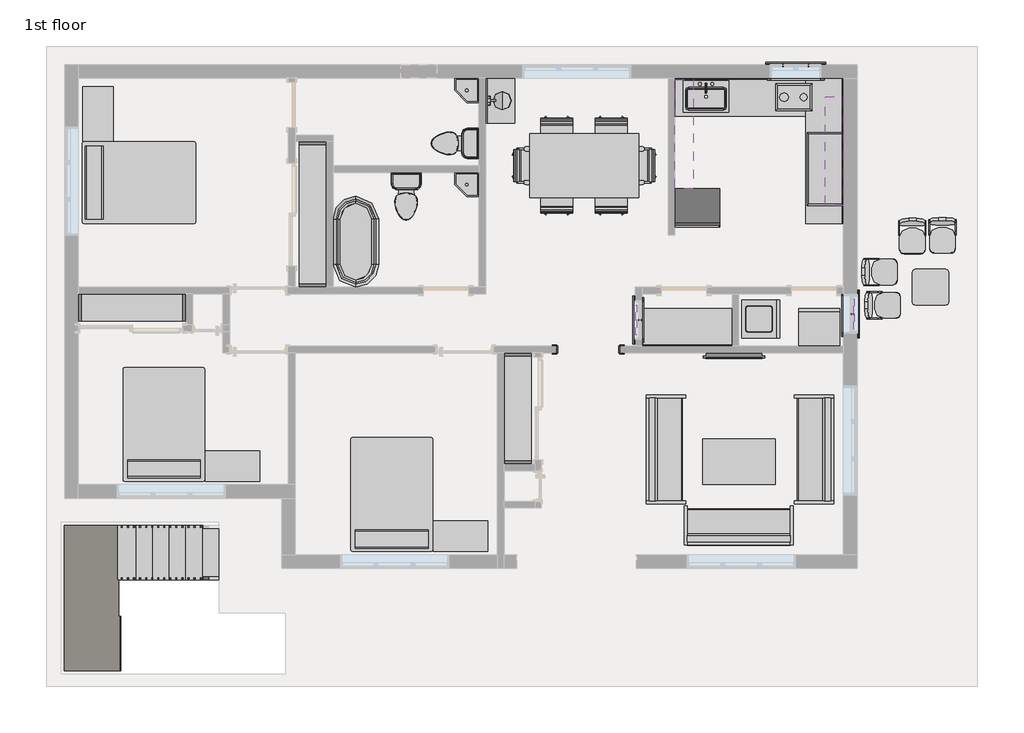
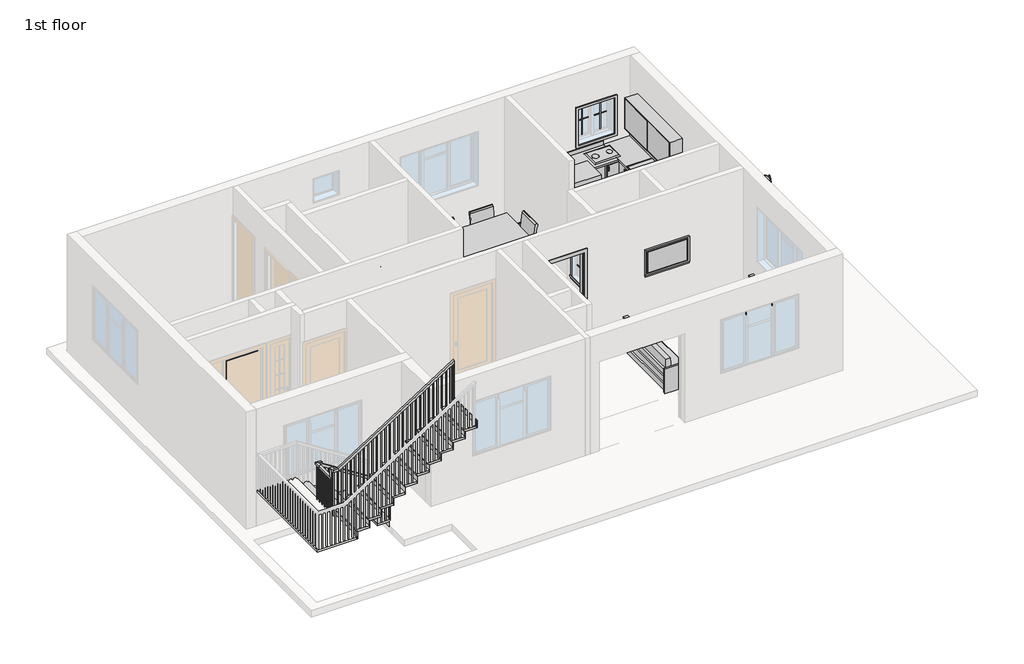
# One storey, part 4 of 4: 34 furniture elements, 17 proxies, 7 flow terminals, 2 stair flights, 1 railing, 1 slab.
"""IFC4 building model written with IfcOpenShell, lengths in millimetres."""

from ifc_helpers import new_model, si_unit, frame, origin, place, context, project, spatial, polyline, outline, extrude, faceted_brep, transform, mapped, element, save
from components import proxy_3c1fa1d0, proxy_97c73763, muntin_pattern_2x2_muntin_pattern_2x2_b3fe6957, muntin_pattern_2x2_muntin_pattern_2x2_3e0ecaf2, muntin_pattern_2x2_muntin_pattern_2x2_c35c595f, muntin_pattern_2x2_muntin_pattern_2x2_183aef24, proxy_bc9927fa, proxy_e6cf46b9, trim_window_exterior_flat_with_sill_41619996, trim_window_exterior_flat_with_sill_e38017c9, trim_window_exterior_flat_with_sill_5e960bf5, trim_window_interior_flat_picture_frame_51c85655, trim_window_interior_flat_picture_frame_d728ed12, trim_window_interior_flat_picture_frame_80babb00, proxy_1934c8a4, flow_terminal_15267b2a, flow_terminal_5b58e753, flow_terminal_4d548711, toilet_domestic_3d_toilet_domestic_3d_ba6479b0, toilet_domestic_3d_toilet_domestic_3d_30431060, flow_terminal_ce36f001, furniture_48488436, furniture_f87f75a4, furniture_97fe820d, furniture_52ef1662, furniture_6b884072, chair_task_chair_task_b7f3823b, chair_task_arms_chair_task_arms_fa5a08ef, furniture_deb1c5d1, furniture_9388d8e7, furniture_74614b7d, furniture_eb3a3c23, furniture_53a00f75, furniture_df918c0e, furniture_57be741f, furniture_57f9710a, furniture_acc2807d, furniture_65ba067b, furniture_5d68651d, furniture_b6aab1a0, furniture_1cc80a06, non_monolithic_landing_2594b9d5, stair_flight_c0af1c60, stair_flight_c577b9fb

model = new_model("IFC4")

# Units and contexts
model_context = context("Model", 3, world=origin())
ifc_project = project(units=[si_unit("LENGTHUNIT", "METRE", prefix="MILLI")], contexts=[model_context])

# Site, building, storey
site = spatial("IfcSite", under=ifc_project)
building = spatial("IfcBuilding", under=site)
storey = spatial("IfcBuildingStorey", under=building, Name="1st floor", Elevation=3810.0)

# Proxies
placement = place(None, origin())
proxy_shape = proxy_3c1fa1d0(model_context)
element("IfcBuildingElementProxy", 1, Name="Cook Top-2 Unit : 12\" x 18\"", ObjectType="Cook Top-2 Unit : 12\" x 18\"", at=placement, inside=storey, context=model_context, shape_type="MappedRepresentation", body=[
    mapped(proxy_shape, transform((3099.7984427, 6060.3661978, 3810.0), x_axis=(0.0, 1.0, 0.0), y_axis=(-1.0, 0.0, 0.0), z_axis=(0.0, 0.0, 1.0))),
])
proxy_2_shape = proxy_97c73763(model_context)
element("IfcBuildingElementProxy", 2, Name="Dryer : 27\" x 25\" x 35\"", ObjectType="Dryer : 27\" x 25\" x 35\"", at=placement, inside=storey, context=model_context, shape_type="MappedRepresentation", body=[
    mapped(proxy_2_shape, transform((3116.0361908, 1961.105194, 3810.0), x_axis=(1.0, 0.0, 0.0), y_axis=(0.0, 1.0, 0.0), z_axis=(0.0, 0.0, 1.0))),
])
muntin_pattern_2x2_muntin_pattern_2x2_shape = muntin_pattern_2x2_muntin_pattern_2x2_b3fe6957(model_context)
element("IfcBuildingElementProxy", 3, Name="Muntin Pattern_2x2 : Muntin Pattern_2x2", ObjectType="Muntin Pattern_2x2 : Muntin Pattern_2x2", at=placement, inside=storey, context=model_context, shape_type="MappedRepresentation", body=[
    mapped(muntin_pattern_2x2_muntin_pattern_2x2_shape, transform((2887.0111471, 6673.1411978, 4972.05), x_axis=(1.0, 0.0, 0.0), y_axis=(0.0, 1.0, 0.0), z_axis=(0.0, 0.0, 1.0))),
])
muntin_pattern_2x2_muntin_pattern_2x2_2_shape = muntin_pattern_2x2_muntin_pattern_2x2_3e0ecaf2(model_context)
element("IfcBuildingElementProxy", 4, Name="Muntin Pattern_2x2 : Muntin Pattern_2x2", ObjectType="Muntin Pattern_2x2 : Muntin Pattern_2x2", at=placement, inside=storey, context=model_context, shape_type="MappedRepresentation", body=[
    mapped(muntin_pattern_2x2_muntin_pattern_2x2_2_shape, transform((3315.6361471, 6673.1411978, 4972.05), x_axis=(-1.0, 0.0, 0.0), y_axis=(0.0, -1.0, 0.0), z_axis=(0.0, 0.0, 1.0))),
])
muntin_pattern_2x2_muntin_pattern_2x2_3_shape = muntin_pattern_2x2_muntin_pattern_2x2_c35c595f(model_context)
element("IfcBuildingElementProxy", 5, Name="Muntin Pattern_2x2 : Muntin Pattern_2x2", ObjectType="Muntin Pattern_2x2 : Muntin Pattern_2x2", at=placement, inside=storey, context=model_context, shape_type="MappedRepresentation", body=[
    mapped(muntin_pattern_2x2_muntin_pattern_2x2_3_shape, transform((4095.0986471, 2498.0161978, 5280.025), x_axis=(0.0, -1.0, 0.0), y_axis=(1.0, 0.0, 0.0), z_axis=(0.0, 0.0, 1.0))),
])
element("IfcBuildingElementProxy", 6, Name="Muntin Pattern_2x2 : Muntin Pattern_2x2", ObjectType="Muntin Pattern_2x2 : Muntin Pattern_2x2", at=placement, inside=storey, context=model_context, shape_type="MappedRepresentation", body=[
    mapped(muntin_pattern_2x2_muntin_pattern_2x2_3_shape, transform((4050.6486471, 2498.0161978, 4800.6), x_axis=(0.0, -1.0, 0.0), y_axis=(1.0, 0.0, 0.0), z_axis=(0.0, 0.0, 1.0))),
])
muntin_pattern_2x2_muntin_pattern_2x2_4_shape = muntin_pattern_2x2_muntin_pattern_2x2_183aef24(model_context)
element("IfcBuildingElementProxy", 7, Name="Muntin Pattern_2x2 : Muntin Pattern_2x2", ObjectType="Muntin Pattern_2x2 : Muntin Pattern_2x2", at=placement, inside=storey, context=model_context, shape_type="MappedRepresentation", body=[
    mapped(muntin_pattern_2x2_muntin_pattern_2x2_4_shape, transform((443.8486471, 2396.4161978, 5280.025), x_axis=(0.0, -1.0, 0.0), y_axis=(1.0, 0.0, 0.0), z_axis=(0.0, 0.0, 1.0))),
])
element("IfcBuildingElementProxy", 8, Name="Muntin Pattern_2x2 : Muntin Pattern_2x2", ObjectType="Muntin Pattern_2x2 : Muntin Pattern_2x2", at=placement, inside=storey, context=model_context, shape_type="MappedRepresentation", body=[
    mapped(muntin_pattern_2x2_muntin_pattern_2x2_4_shape, transform((488.2986471, 2396.4161978, 4800.6), x_axis=(0.0, -1.0, 0.0), y_axis=(1.0, 0.0, 0.0), z_axis=(0.0, 0.0, 1.0))),
])
proxy_3_shape = proxy_bc9927fa(model_context)
element("IfcBuildingElementProxy", 9, Name="Passage Opening-Cased : 36\" x 84\"", ObjectType="Passage Opening-Cased : 36\" x 84\"", at=placement, inside=storey, context=model_context, shape_type="MappedRepresentation", body=[
    mapped(proxy_3_shape, transform((-386.6650096, 1901.1161978, 3810.0), x_axis=(-1.0, 0.0, 0.0), y_axis=(0.0, -1.0, 0.0), z_axis=(0.0, 0.0, 1.0))),
])
proxy_4_shape = proxy_e6cf46b9(model_context)
element("IfcBuildingElementProxy", 10, Name="Refrigerator-Built-in : 30\" x 24\" RH", ObjectType="Refrigerator-Built-in : 30\" x 24\" RH", at=placement, inside=storey, context=model_context, shape_type="MappedRepresentation", body=[
    mapped(proxy_4_shape, transform((1450.3236471, 4309.7422263, 3810.0), x_axis=(1.0, 0.0, 0.0), y_axis=(0.0, 1.0, 0.0), z_axis=(0.0, 0.0, 1.0))),
])
trim_window_exterior_flat_with_sill_shape = trim_window_exterior_flat_with_sill_41619996(model_context)
element("IfcBuildingElementProxy", 11, Name="Trim-Window-Exterior-Flat : with Sill", ObjectType="Trim-Window-Exterior-Flat : with Sill", at=placement, inside=storey, context=model_context, shape_type="MappedRepresentation", body=[
    mapped(trim_window_exterior_flat_with_sill_shape, transform((3101.3236471, 6682.6661978, 5816.6), x_axis=(-1.0, 0.0, 0.0), y_axis=(0.0, 0.0, 1.0), z_axis=(0.0, 1.0, 0.0))),
])
trim_window_exterior_flat_with_sill_2_shape = trim_window_exterior_flat_with_sill_e38017c9(model_context)
element("IfcBuildingElementProxy", 12, Name="Trim-Window-Exterior-Flat : with Sill", ObjectType="Trim-Window-Exterior-Flat : with Sill", at=placement, inside=storey, context=model_context, shape_type="MappedRepresentation", body=[
    mapped(trim_window_exterior_flat_with_sill_2_shape, transform((4130.0236471, 2498.0161978, 5791.2), x_axis=(0.0, 1.0, 0.0), y_axis=(0.0, 0.0, 1.0), z_axis=(1.0, 0.0, 0.0))),
])
trim_window_exterior_flat_with_sill_3_shape = trim_window_exterior_flat_with_sill_5e960bf5(model_context)
element("IfcBuildingElementProxy", 13, Name="Trim-Window-Exterior-Flat : with Sill", ObjectType="Trim-Window-Exterior-Flat : with Sill", at=placement, inside=storey, context=model_context, shape_type="MappedRepresentation", body=[
    mapped(trim_window_exterior_flat_with_sill_3_shape, transform((408.9236471, 2396.4161978, 5791.2), x_axis=(0.0, 1.0, 0.0), y_axis=(0.0, 0.0, -1.0), z_axis=(-1.0, 0.0, 0.0))),
])
trim_window_interior_flat_picture_frame_shape = trim_window_interior_flat_picture_frame_51c85655(model_context)
element("IfcBuildingElementProxy", 14, Name="Trim-Window-Interior-Flat : Picture Frame", ObjectType="Trim-Window-Interior-Flat : Picture Frame", at=placement, inside=storey, context=model_context, shape_type="MappedRepresentation", body=[
    mapped(trim_window_interior_flat_picture_frame_shape, transform((3101.3236471, 6454.0661978, 5816.6), x_axis=(1.0, 0.0, 0.0), y_axis=(0.0, 0.0, 1.0), z_axis=(0.0, -1.0, 0.0))),
])
trim_window_interior_flat_picture_frame_2_shape = trim_window_interior_flat_picture_frame_d728ed12(model_context)
element("IfcBuildingElementProxy", 15, Name="Trim-Window-Interior-Flat : Picture Frame", ObjectType="Trim-Window-Interior-Flat : Picture Frame", at=placement, inside=storey, context=model_context, shape_type="MappedRepresentation", body=[
    mapped(trim_window_interior_flat_picture_frame_2_shape, transform((3901.4236471, 2498.0161978, 5791.2), x_axis=(0.0, -1.0, 0.0), y_axis=(0.0, 0.0, 1.0), z_axis=(-1.0, 0.0, 0.0))),
])
trim_window_interior_flat_picture_frame_3_shape = trim_window_interior_flat_picture_frame_80babb00(model_context)
element("IfcBuildingElementProxy", 16, Name="Trim-Window-Interior-Flat : Picture Frame", ObjectType="Trim-Window-Interior-Flat : Picture Frame", at=placement, inside=storey, context=model_context, shape_type="MappedRepresentation", body=[
    mapped(trim_window_interior_flat_picture_frame_3_shape, transform((523.2236471, 2396.4161978, 5791.2), x_axis=(0.0, -1.0, 0.0), y_axis=(0.0, 0.0, -1.0), z_axis=(1.0, 0.0, 0.0))),
])
proxy_5_shape = proxy_1934c8a4(model_context)
element("IfcBuildingElementProxy", 17, Name="Washer : 25\" x 25\" x 35\"", ObjectType="Washer : 25\" x 25\" x 35\"", at=placement, inside=storey, context=model_context, shape_type="MappedRepresentation", body=[
    mapped(proxy_5_shape, transform((2237.9740823, 2809.1661978, 3810.0), x_axis=(0.0, -1.0, 0.0), y_axis=(1.0, 0.0, 0.0), z_axis=(0.0, 0.0, 1.0))),
])

# Flow terminals
flow_terminal_shape = flow_terminal_15267b2a(model_context)
element("IfcFlowTerminal", 18, ObjectType="Lavatory - Vanity : 30\"x18\" - Private", at=placement, inside=storey, context=model_context, shape_type="MappedRepresentation", body=[
    mapped(flow_terminal_shape, transform((-2099.3263529, 6079.4161978, 3810.0), x_axis=(1.0, 0.0, 0.0), y_axis=(0.0, 1.0, 0.0), z_axis=(0.0, 0.0, 1.0))),
])
flow_terminal_2_shape = flow_terminal_5b58e753(model_context)
element("IfcFlowTerminal", 19, ObjectType="Sink - Mop : 28\"x28\"", at=placement, inside=storey, context=model_context, shape_type="MappedRepresentation", body=[
    mapped(flow_terminal_2_shape, transform((-2213.6263529, 4872.9161978, 3810.0), x_axis=(0.0, -1.0, 0.0), y_axis=(1.0, 0.0, 0.0), z_axis=(0.0, 0.0, 1.0))),
])
element("IfcFlowTerminal", 20, ObjectType="Sink - Mop : 28\"x28\"", at=placement, inside=storey, context=model_context, shape_type="MappedRepresentation", body=[
    mapped(flow_terminal_2_shape, transform((-2213.6263529, 6454.0661978, 3810.0), x_axis=(0.0, -1.0, 0.0), y_axis=(1.0, 0.0, 0.0), z_axis=(0.0, 0.0, 1.0))),
])
flow_terminal_3_shape = flow_terminal_4d548711(model_context)
element("IfcFlowTerminal", 21, ObjectType="Sink Kitchen-Single : 30\" x 21\"", at=placement, inside=storey, context=model_context, shape_type="MappedRepresentation", body=[
    mapped(flow_terminal_3_shape, transform((1580.6844065, 6146.9207967, 3810.0), x_axis=(1.0, 0.0, 0.0), y_axis=(0.0, 1.0, 0.0), z_axis=(0.0, 0.0, 1.0))),
])
toilet_domestic_3d_toilet_domestic_3d_shape = toilet_domestic_3d_toilet_domestic_3d_ba6479b0(model_context)
toilet_domestic_3d_toilet_domestic_3d_2_shape = toilet_domestic_3d_toilet_domestic_3d_30431060(model_context)
element("IfcFlowTerminal", 22, ObjectType="Toilet-Domestic-3D : Toilet-Domestic-3D", at=placement, inside=storey, context=model_context, shape_type="MappedRepresentation", body=[
    mapped(toilet_domestic_3d_toilet_domestic_3d_shape, transform((-3433.7493286, 4378.2201704, 3810.0), x_axis=(1.0, 0.0, 0.0), y_axis=(0.0, 1.0, 0.0), z_axis=(0.0, 0.0, 1.0))),
    mapped(toilet_domestic_3d_toilet_domestic_3d_2_shape, transform((-3433.7493286, 4378.2201704, 3810.0), x_axis=(1.0, 0.0, 0.0), y_axis=(0.0, 1.0, 0.0), z_axis=(0.0, 0.0, 1.0))),
])
element("IfcFlowTerminal", 23, ObjectType="Toilet-Domestic-3D : Toilet-Domestic-3D", at=placement, inside=storey, context=model_context, shape_type="MappedRepresentation", body=[
    mapped(toilet_domestic_3d_toilet_domestic_3d_shape, transform((-2708.3223803, 5361.8661978, 3810.0), x_axis=(0.0, -1.0, 0.0), y_axis=(1.0, 0.0, 0.0), z_axis=(0.0, 0.0, 1.0))),
    mapped(toilet_domestic_3d_toilet_domestic_3d_2_shape, transform((-2708.3223803, 5361.8661978, 3810.0), x_axis=(0.0, -1.0, 0.0), y_axis=(1.0, 0.0, 0.0), z_axis=(0.0, 0.0, 1.0))),
])
flow_terminal_4_shape = flow_terminal_ce36f001(model_context)
element("IfcFlowTerminal", 24, ObjectType="Tub-Free Standing-3D : 30\" x 60\"", at=placement, inside=storey, context=model_context, shape_type="MappedRepresentation", body=[
    mapped(flow_terminal_4_shape, transform((-4277.3763529, 3710.8661978, 3810.0), x_axis=(-1.0, 0.0, 0.0), y_axis=(0.0, -1.0, 0.0), z_axis=(0.0, 0.0, 1.0))),
])

# Furniture
furniture_shape = furniture_48488436(model_context)
element("IfcFurniture", 25, ObjectType="48\"", at=placement, inside=storey, context=model_context, shape_type="MappedRepresentation", body=[
    mapped(furniture_shape, transform((3901.4236471, 5020.9111578, 3810.0), x_axis=(0.0, -1.0, 0.0), y_axis=(1.0, 0.0, 0.0), z_axis=(0.0, 0.0, 1.0))),
])
furniture_2_shape = furniture_f87f75a4(model_context)
element("IfcFurniture", 26, ObjectType="Base Cabinet-Combo01 : 30\"", at=placement, inside=storey, context=model_context, shape_type="MappedRepresentation", body=[
    mapped(furniture_2_shape, transform((2587.2859422, 6454.0661978, 3810.0), x_axis=(1.0, 0.0, 0.0), y_axis=(0.0, 1.0, 0.0), z_axis=(0.0, 0.0, 1.0))),
])
furniture_3_shape = furniture_97fe820d(model_context)
element("IfcFurniture", 27, ObjectType="Base Cabinet-Corner Unit-Square : 36\"", at=placement, inside=storey, context=model_context, shape_type="MappedRepresentation", body=[
    mapped(furniture_3_shape, transform((3374.6859422, 6454.0661978, 3810.0), x_axis=(1.0, 0.0, 0.0), y_axis=(0.0, 1.0, 0.0), z_axis=(0.0, 0.0, 1.0))),
])
furniture_4_shape = furniture_52ef1662(model_context)
element("IfcFurniture", 28, ObjectType="Bed-Standard : Double 54\" x 75\"", at=placement, inside=storey, context=model_context, shape_type="MappedRepresentation", body=[
    mapped(furniture_4_shape, transform((-7961.5214349, 4429.9776732, 3810.0), x_axis=(0.0, 1.0, 0.0), y_axis=(-1.0, 0.0, 0.0), z_axis=(0.0, 0.0, 1.0))),
])
element("IfcFurniture", 29, ObjectType="Bed-Standard : Double 54\" x 75\"", at=placement, inside=storey, context=model_context, shape_type="MappedRepresentation", body=[
    mapped(furniture_4_shape, transform((-7225.3378283, 598.2211158, 3810.0), x_axis=(-1.0, 0.0, 0.0), y_axis=(0.0, -1.0, 0.0), z_axis=(0.0, 0.0, 1.0))),
])
element("IfcFurniture", 30, ObjectType="Bed-Standard : Double 54\" x 75\"", at=placement, inside=storey, context=model_context, shape_type="MappedRepresentation", body=[
    mapped(furniture_4_shape, transform((-3402.6378283, -576.5288842, 3810.0), x_axis=(-1.0, 0.0, 0.0), y_axis=(0.0, -1.0, 0.0), z_axis=(0.0, 0.0, 1.0))),
])
furniture_5_shape = furniture_6b884072(model_context)
element("IfcFurniture", 31, ObjectType="Cabinet File-Lateral 2 Drawer : 36\" x 20\" x 24\"", at=placement, inside=storey, context=model_context, shape_type="MappedRepresentation", body=[
    mapped(furniture_5_shape, transform((-9536.044729, 6037.1887117, 3810.0), x_axis=(0.0, 1.0, 0.0), y_axis=(-1.0, 0.0, 0.0), z_axis=(0.0, 0.0, 1.0))),
])
element("IfcFurniture", 32, ObjectType="Cabinet File-Lateral 2 Drawer : 36\" x 20\" x 24\"", at=placement, inside=storey, context=model_context, shape_type="MappedRepresentation", body=[
    mapped(furniture_5_shape, transform((-6527.4988668, -989.0021783, 3810.0), x_axis=(-1.0, 0.0, 0.0), y_axis=(0.0, -1.0, 0.0), z_axis=(0.0, 0.0, 1.0))),
])
element("IfcFurniture", 33, ObjectType="Cabinet File-Lateral 2 Drawer : 36\" x 20\" x 24\"", at=placement, inside=storey, context=model_context, shape_type="MappedRepresentation", body=[
    mapped(furniture_5_shape, transform((-2698.4488668, -2163.7521783, 3810.0), x_axis=(-1.0, 0.0, 0.0), y_axis=(0.0, -1.0, 0.0), z_axis=(0.0, 0.0, 1.0))),
])
chair_task_chair_task_shape = chair_task_chair_task_b7f3823b(model_context)
element("IfcFurniture", 34, ObjectType="Chair-Task : Chair-Task", at=placement, inside=storey, context=model_context, shape_type="MappedRepresentation", body=[
    mapped(chair_task_chair_task_shape, transform((149.8644668, 5539.5620994, 3810.0), x_axis=(-1.0, 0.0, 0.0), y_axis=(0.0, -1.0, 0.0), z_axis=(0.0, 0.0, 1.0))),
])
element("IfcFurniture", 35, ObjectType="Chair-Task : Chair-Task", at=placement, inside=storey, context=model_context, shape_type="MappedRepresentation", body=[
    mapped(chair_task_chair_task_shape, transform((-132.1171726, 4434.8702962, 3810.0), x_axis=(1.0, 0.0, 0.0), y_axis=(0.0, 1.0, 0.0), z_axis=(0.0, 0.0, 1.0))),
])
element("IfcFurniture", 36, ObjectType="Chair-Task : Chair-Task", at=placement, inside=storey, context=model_context, shape_type="MappedRepresentation", body=[
    mapped(chair_task_chair_task_shape, transform((-764.5355332, 5539.5620994, 3810.0), x_axis=(-1.0, 0.0, 0.0), y_axis=(0.0, -1.0, 0.0), z_axis=(0.0, 0.0, 1.0))),
])
element("IfcFurniture", 37, ObjectType="Chair-Task : Chair-Task", at=placement, inside=storey, context=model_context, shape_type="MappedRepresentation", body=[
    mapped(chair_task_chair_task_shape, transform((-1046.5171726, 4434.8702962, 3810.0), x_axis=(1.0, 0.0, 0.0), y_axis=(0.0, 1.0, 0.0), z_axis=(0.0, 0.0, 1.0))),
])
chair_task_arms_chair_task_arms_shape = chair_task_arms_chair_task_arms_fa5a08ef(model_context)
element("IfcFurniture", 38, ObjectType="Chair-Task Arms : Chair-Task Arms", at=placement, inside=storey, context=model_context, shape_type="MappedRepresentation", body=[
    mapped(chair_task_arms_chair_task_arms_shape, transform((-1381.6722545, 5128.2070175, 3810.0), x_axis=(0.0, -1.0, 0.0), y_axis=(1.0, 0.0, 0.0), z_axis=(0.0, 0.0, 1.0))),
])
element("IfcFurniture", 39, ObjectType="Chair-Task Arms : Chair-Task Arms", at=placement, inside=storey, context=model_context, shape_type="MappedRepresentation", body=[
    mapped(chair_task_arms_chair_task_arms_shape, transform((485.0195487, 4846.2253781, 3810.0), x_axis=(0.0, 1.0, 0.0), y_axis=(-1.0, 0.0, 0.0), z_axis=(0.0, 0.0, 1.0))),
])
furniture_6_shape = furniture_deb1c5d1(model_context)
element("IfcFurniture", 40, ObjectType="Counter Top : 24\" Depth", at=placement, inside=storey, context=model_context, shape_type="MappedRepresentation", body=[
    mapped(furniture_6_shape, transform((3901.4236471, 5253.6039027, 3810.0), x_axis=(0.0, -1.0, 0.0), y_axis=(1.0, 0.0, 0.0), z_axis=(0.0, 0.0, 1.0))),
])
furniture_7_shape = furniture_9388d8e7(model_context)
element("IfcFurniture", 41, ObjectType="Counter Top : 24\" Depth", at=placement, inside=storey, context=model_context, shape_type="MappedRepresentation", body=[
    mapped(furniture_7_shape, transform((834.061352, 1958.2661978, 3810.0), x_axis=(-1.0, 0.0, 0.0), y_axis=(0.0, -1.0, 0.0), z_axis=(0.0, 0.0, 1.0))),
])
furniture_8_shape = furniture_74614b7d(model_context)
element("IfcFurniture", 42, ObjectType="Counter Top w Sink Hole : 24\" Depth", at=placement, inside=storey, context=model_context, shape_type="MappedRepresentation", body=[
    mapped(furniture_8_shape, transform((2276.1359422, 6454.0661978, 3810.0), x_axis=(1.0, 0.0, 0.0), y_axis=(0.0, 1.0, 0.0), z_axis=(0.0, 0.0, 1.0))),
])
furniture_9_shape = furniture_eb3a3c23(model_context)
element("IfcFurniture", 43, ObjectType="Seating-Auditorium : 18\" x 24\" x 30\"", at=placement, inside=storey, context=model_context, shape_type="MappedRepresentation", body=[
    mapped(furniture_9_shape, transform((4308.4482373, 3363.5940666, 3810.0), x_axis=(0.0, -1.0, 0.0), y_axis=(1.0, 0.0, 0.0), z_axis=(0.0, 0.0, 1.0))),
])
element("IfcFurniture", 44, ObjectType="Seating-Auditorium : 18\" x 24\" x 30\"", at=placement, inside=storey, context=model_context, shape_type="MappedRepresentation", body=[
    mapped(furniture_9_shape, transform((4359.2482373, 2804.7940666, 3810.0), x_axis=(0.0, -1.0, 0.0), y_axis=(1.0, 0.0, 0.0), z_axis=(0.0, 0.0, 1.0))),
])
element("IfcFurniture", 45, ObjectType="Seating-Auditorium : 18\" x 24\" x 30\"", at=placement, inside=storey, context=model_context, shape_type="MappedRepresentation", body=[
    mapped(furniture_9_shape, transform((5217.8515159, 4002.3416076, 3810.0), x_axis=(-1.0, 0.0, 0.0), y_axis=(0.0, -1.0, 0.0), z_axis=(0.0, 0.0, 1.0))),
])
element("IfcFurniture", 46, ObjectType="Seating-Auditorium : 18\" x 24\" x 30\"", at=placement, inside=storey, context=model_context, shape_type="MappedRepresentation", body=[
    mapped(furniture_9_shape, transform((5725.8515159, 4015.0416076, 3810.0), x_axis=(-1.0, 0.0, 0.0), y_axis=(0.0, -1.0, 0.0), z_axis=(0.0, 0.0, 1.0))),
])
furniture_10_shape = furniture_53a00f75(model_context)
element("IfcFurniture", 47, ObjectType="Shelving : 96\" x 12\" x 84\"", at=placement, inside=storey, context=model_context, shape_type="MappedRepresentation", body=[
    mapped(furniture_10_shape, transform((-1864.3763529, 910.5161978, 3810.0), x_axis=(0.0, 1.0, 0.0), y_axis=(-1.0, 0.0, 0.0), z_axis=(0.0, 0.0, 1.0))),
])
furniture_11_shape = furniture_df918c0e(model_context)
element("IfcFurniture", 48, ObjectType="Shelving : 96\" x 12\" x 84\" 2", at=placement, inside=storey, context=model_context, shape_type="MappedRepresentation", body=[
    mapped(furniture_11_shape, transform((-8030.2263529, 2910.7661978, 3810.0), x_axis=(1.0, 0.0, 0.0), y_axis=(0.0, 1.0, 0.0), z_axis=(0.0, 0.0, 1.0))),
])
furniture_12_shape = furniture_57be741f(model_context)
element("IfcFurniture", 49, ObjectType="Shelving : 96\" x 12\" x 84\" 3", at=placement, inside=storey, context=model_context, shape_type="MappedRepresentation", body=[
    mapped(furniture_12_shape, transform((-5306.0763529, 4168.0661978, 3810.0), x_axis=(0.0, 1.0, 0.0), y_axis=(-1.0, 0.0, 0.0), z_axis=(0.0, 0.0, 1.0))),
])
furniture_13_shape = furniture_57f9710a(model_context)
element("IfcFurniture", 50, ObjectType="Sofa : 72\"", at=placement, inside=storey, context=model_context, shape_type="MappedRepresentation", body=[
    mapped(furniture_13_shape, transform((2219.1941389, -905.4797038, 3810.0), x_axis=(-1.0, 0.0, 0.0), y_axis=(0.0, -1.0, 0.0), z_axis=(0.0, 0.0, 1.0))),
])
element("IfcFurniture", 51, ObjectType="Sofa : 72\"", at=placement, inside=storey, context=model_context, shape_type="MappedRepresentation", body=[
    mapped(furniture_13_shape, transform((3259.9695487, 295.0866896, 3810.0), x_axis=(0.0, -1.0, 0.0), y_axis=(1.0, 0.0, 0.0), z_axis=(0.0, 0.0, 1.0))),
])
element("IfcFurniture", 52, ObjectType="Sofa : 72\"", at=placement, inside=storey, context=model_context, shape_type="MappedRepresentation", body=[
    mapped(furniture_13_shape, transform((1069.4277455, 154.345706, 3810.0), x_axis=(0.0, 1.0, 0.0), y_axis=(-1.0, 0.0, 0.0), z_axis=(0.0, 0.0, 1.0))),
])
furniture_14_shape = furniture_acc2807d(model_context)
element("IfcFurniture", 53, ObjectType="Table-Coffee Rectangular : 48\" x 30\"", at=placement, inside=storey, context=model_context, shape_type="MappedRepresentation", body=[
    mapped(furniture_14_shape, transform((1535.4900168, -354.444634, 3810.0), x_axis=(1.0, 0.0, 0.0), y_axis=(0.0, 1.0, 0.0), z_axis=(0.0, 0.0, 1.0))),
])
furniture_15_shape = furniture_65ba067b(model_context)
element("IfcFurniture", 54, ObjectType="Table-Conference2 w Chairs : 40\" x 90\"", at=placement, inside=storey, context=model_context, shape_type="MappedRepresentation", body=[
    mapped(furniture_15_shape, transform((-448.3263529, 4987.2161978, 3810.0), x_axis=(1.0, 0.0, 0.0), y_axis=(0.0, 1.0, 0.0), z_axis=(0.0, 0.0, 1.0))),
])
furniture_16_shape = furniture_5d68651d(model_context)
element("IfcFurniture", 55, ObjectType="Table-End : 24\" x 24\"", at=placement, inside=storey, context=model_context, shape_type="MappedRepresentation", body=[
    mapped(furniture_16_shape, transform((5053.3900168, 2796.4661978, 3810.0), x_axis=(1.0, 0.0, 0.0), y_axis=(0.0, 1.0, 0.0), z_axis=(0.0, 0.0, 1.0))),
])
furniture_17_shape = furniture_b6aab1a0(model_context)
element("IfcFurniture", 56, ObjectType="Television-Plasma : 42\"", at=placement, inside=storey, context=model_context, shape_type="MappedRepresentation", body=[
    mapped(furniture_17_shape, transform((2009.1236471, 1843.9661978, 4876.8), x_axis=(1.0, 0.0, 0.0), y_axis=(0.0, 1.0, 0.0), z_axis=(0.0, 0.0, 1.0))),
])
furniture_18_shape = furniture_1cc80a06(model_context)
element("IfcFurniture", 57, ObjectType="Upper Cabinet-Pass-Thru w Glass : 48\" x 30\" x 12\"", at=placement, inside=storey, context=model_context, shape_type="MappedRepresentation", body=[
    mapped(furniture_18_shape, transform((1075.6736471, 5495.5284929, 3810.0), x_axis=(0.0, 1.0, 0.0), y_axis=(-1.0, 0.0, 0.0), z_axis=(0.0, 0.0, 1.0))),
])
element("IfcFurniture", 58, ObjectType="Upper Cabinet-Pass-Thru w Glass : 48\" x 30\" x 12\"", at=placement, inside=storey, context=model_context, shape_type="MappedRepresentation", body=[
    mapped(furniture_18_shape, transform((3596.6236471, 5216.1284929, 3810.0), x_axis=(0.0, 1.0, 0.0), y_axis=(-1.0, 0.0, 0.0), z_axis=(0.0, 0.0, 1.0))),
])

# Railing
element("IfcRailing", 59, ObjectType="Handrail - Rectangular", at=placement, inside=storey, context=model_context, shape_type="SolidModel", body=[
    faceted_brep([(-6576.0763529, -1966.0338022, 4902.2), (-6576.0763529, -1966.0338022, 4841.986276), (-6576.0763529, -1915.2338022, 4841.986276), (-6576.0763529, -1915.2338022, 4902.2), (-8176.2763529, -1966.0338022, 5920.5090909), (-8227.0763529, -1966.0338022, 5892.6226396), (-8227.0763529, -1915.2338022, 5892.6226396), (-8176.2763529, -1915.2338022, 5920.5090909), (-8176.2763529, -1966.0338022, 5969.0), (-8227.0763529, -1966.0338022, 5918.2), (-8227.0763529, -1915.2338022, 5918.2), (-8176.2763529, -1915.2338022, 5969.0), (-8252.4763529, -1966.0338022, 5969.0), (-8252.4763529, -1966.0338022, 5918.2), (-8303.2763529, -1915.2338022, 5918.2), (-8303.2763529, -1915.2338022, 5969.0), (-8252.4763529, -2042.2338022, 5969.0), (-8252.4763529, -2042.2338022, 5918.2), (-8303.2763529, -2042.2338022, 5918.2), (-8303.2763529, -2042.2338022, 5969.0), (-8252.4763529, -2499.4338022, 5969.0), (-8252.4763529, -2550.2338022, 5918.2), (-8303.2763529, -2550.2338022, 5918.2), (-8303.2763529, -2499.4338022, 5969.0), (-8252.4763529, -2499.4338022, 6195.2909091), (-8252.4763529, -2550.2338022, 6144.4909091), (-8303.2763529, -2550.2338022, 6144.4909091), (-8303.2763529, -2499.4338022, 6195.2909091), (-8252.4763529, -2575.6338022, 6195.2909091), (-8252.4763529, -2575.6338022, 6144.4909091), (-8303.2763529, -2626.4338022, 6144.4909091), (-8303.2763529, -2626.4338022, 6195.2909091), (-8176.2763529, -2575.6338022, 6195.2909091), (-8161.483358, -2575.6338022, 6144.4909091), (-8161.483358, -2626.4338022, 6144.4909091), (-8176.2763529, -2626.4338022, 6195.2909091), (-5458.4763529, -2575.6338022, 7924.8), (-5458.4763529, -2626.4338022, 7924.8), (-5458.4763529, -2626.4338022, 7864.586276), (-5458.4763529, -2575.6338022, 7864.586276)], [[[0, 1, 2, 3]], [[1, 0, 4, 5]], [[2, 1, 5, 6]], [[3, 2, 6, 7]], [[0, 3, 7, 4]], [[5, 4, 8, 9]], [[6, 5, 9, 10]], [[7, 6, 10, 11]], [[4, 7, 11, 8]], [[9, 8, 12, 13]], [[10, 9, 13, 14]], [[11, 10, 14, 15]], [[8, 11, 15, 12]], [[13, 12, 16, 17]], [[14, 13, 17, 18]], [[15, 14, 18, 19]], [[12, 15, 19, 16]], [[17, 16, 20, 21]], [[18, 17, 21, 22]], [[19, 18, 22, 23]], [[16, 19, 23, 20]], [[21, 20, 24, 25]], [[22, 21, 25, 26]], [[23, 22, 26, 27]], [[20, 23, 27, 24]], [[25, 24, 28, 29]], [[26, 25, 29, 30]], [[27, 26, 30, 31]], [[24, 27, 31, 28]], [[29, 28, 32, 33]], [[30, 29, 33, 34]], [[31, 30, 34, 35]], [[28, 31, 35, 32]], [[36, 37, 38, 39]], [[33, 32, 36, 39]], [[34, 33, 39, 38]], [[35, 34, 38, 37]], [[32, 35, 37, 36]]]),
    extrude(outline(polyline([(7810.0340032, -5544.2013529), (6832.6, -5544.2013529), (6832.6, -5525.1513529), (7822.1567305, -5525.1513529), (7810.0340032, -5544.2013529)])), frame((0.0, -2610.5588022, 0.0), z_axis=(0.0, 1.0, 0.0), x_axis=(0.0, 0.0, 1.0)), (0.0, 0.0, 1.0), 19.05),
    extrude(outline(polyline([(7745.3794578, -5645.8013529), (6832.6, -5645.8013529), (6832.6, -5626.7513529), (7757.5021851, -5626.7513529), (7745.3794578, -5645.8013529)])), frame((0.0, -2610.5588022, 0.0), z_axis=(0.0, 1.0, 0.0), x_axis=(0.0, 0.0, 1.0)), (0.0, 0.0, 1.0), 19.05),
    extrude(outline(polyline([(7680.7249123, -5747.4013529), (6832.6, -5747.4013529), (6832.6, -5728.3513529), (7692.8476396, -5728.3513529), (7680.7249123, -5747.4013529)])), frame((0.0, -2610.5588022, 0.0), z_axis=(0.0, 1.0, 0.0), x_axis=(0.0, 0.0, 1.0)), (0.0, 0.0, 1.0), 19.05),
    extrude(outline(polyline([(7616.0703669, -5849.0013529), (6654.8, -5849.0013529), (6654.8, -5829.9513529), (7628.1930941, -5829.9513529), (7616.0703669, -5849.0013529)])), frame((0.0, -2610.5588022, 0.0), z_axis=(0.0, 1.0, 0.0), x_axis=(0.0, 0.0, 1.0)), (0.0, 0.0, 1.0), 19.05),
    extrude(outline(polyline([(7551.4158214, -5950.6013529), (6654.8, -5950.6013529), (6654.8, -5931.5513529), (7563.5385487, -5931.5513529), (7551.4158214, -5950.6013529)])), frame((0.0, -2610.5588022, 0.0), z_axis=(0.0, 1.0, 0.0), x_axis=(0.0, 0.0, 1.0)), (0.0, 0.0, 1.0), 19.05),
    extrude(outline(polyline([(7486.761276, -6052.2013529), (6477.0, -6052.2013529), (6477.0, -6033.1513529), (7498.8840032, -6033.1513529), (7486.761276, -6052.2013529)])), frame((0.0, -2610.5588022, 0.0), z_axis=(0.0, 1.0, 0.0), x_axis=(0.0, 0.0, 1.0)), (0.0, 0.0, 1.0), 19.05),
    extrude(outline(polyline([(7422.1067305, -6153.8013529), (6477.0, -6153.8013529), (6477.0, -6134.7513529), (7434.2294578, -6134.7513529), (7422.1067305, -6153.8013529)])), frame((0.0, -2610.5588022, 0.0), z_axis=(0.0, 1.0, 0.0), x_axis=(0.0, 0.0, 1.0)), (0.0, 0.0, 1.0), 19.05),
    extrude(outline(polyline([(7357.4521851, -6255.4013529), (6477.0, -6255.4013529), (6477.0, -6236.3513529), (7369.5749123, -6236.3513529), (7357.4521851, -6255.4013529)])), frame((0.0, -2610.5588022, 0.0), z_axis=(0.0, 1.0, 0.0), x_axis=(0.0, 0.0, 1.0)), (0.0, 0.0, 1.0), 19.05),
    extrude(outline(polyline([(7292.7976396, -6357.0013529), (6299.2, -6357.0013529), (6299.2, -6337.9513529), (7304.9203669, -6337.9513529), (7292.7976396, -6357.0013529)])), frame((0.0, -2610.5588022, 0.0), z_axis=(0.0, 1.0, 0.0), x_axis=(0.0, 0.0, 1.0)), (0.0, 0.0, 1.0), 19.05),
    extrude(outline(polyline([(7228.1430941, -6458.6013529), (6299.2, -6458.6013529), (6299.2, -6439.5513529), (7240.2658214, -6439.5513529), (7228.1430941, -6458.6013529)])), frame((0.0, -2610.5588022, 0.0), z_axis=(0.0, 1.0, 0.0), x_axis=(0.0, 0.0, 1.0)), (0.0, 0.0, 1.0), 19.05),
    extrude(outline(polyline([(7163.4885487, -6560.2013529), (6299.2, -6560.2013529), (6299.2, -6541.1513529), (7175.611276, -6541.1513529), (7163.4885487, -6560.2013529)])), frame((0.0, -2610.5588022, 0.0), z_axis=(0.0, 1.0, 0.0), x_axis=(0.0, 0.0, 1.0)), (0.0, 0.0, 1.0), 19.05),
    extrude(outline(polyline([(7098.8340032, -6661.8013529), (6121.4, -6661.8013529), (6121.4, -6642.7513529), (7110.9567305, -6642.7513529), (7098.8340032, -6661.8013529)])), frame((0.0, -2610.5588022, 0.0), z_axis=(0.0, 1.0, 0.0), x_axis=(0.0, 0.0, 1.0)), (0.0, 0.0, 1.0), 19.05),
    extrude(outline(polyline([(7034.1794578, -6763.4013529), (6121.4, -6763.4013529), (6121.4, -6744.3513529), (7046.3021851, -6744.3513529), (7034.1794578, -6763.4013529)])), frame((0.0, -2610.5588022, 0.0), z_axis=(0.0, 1.0, 0.0), x_axis=(0.0, 0.0, 1.0)), (0.0, 0.0, 1.0), 19.05),
    extrude(outline(polyline([(6969.5249123, -6865.0013529), (6121.4, -6865.0013529), (6121.4, -6845.9513529), (6981.6476396, -6845.9513529), (6969.5249123, -6865.0013529)])), frame((0.0, -2610.5588022, 0.0), z_axis=(0.0, 1.0, 0.0), x_axis=(0.0, 0.0, 1.0)), (0.0, 0.0, 1.0), 19.05),
    extrude(outline(polyline([(6904.8703669, -6966.6013529), (5943.6, -6966.6013529), (5943.6, -6947.5513529), (6916.9930941, -6947.5513529), (6904.8703669, -6966.6013529)])), frame((0.0, -2610.5588022, 0.0), z_axis=(0.0, 1.0, 0.0), x_axis=(0.0, 0.0, 1.0)), (0.0, 0.0, 1.0), 19.05),
    extrude(outline(polyline([(6840.2158214, -7068.2013529), (5943.6, -7068.2013529), (5943.6, -7049.1513529), (6852.3385487, -7049.1513529), (6840.2158214, -7068.2013529)])), frame((0.0, -2610.5588022, 0.0), z_axis=(0.0, 1.0, 0.0), x_axis=(0.0, 0.0, 1.0)), (0.0, 0.0, 1.0), 19.05),
    extrude(outline(polyline([(6775.561276, -7169.8013529), (5765.8, -7169.8013529), (5765.8, -7150.7513529), (6787.6840032, -7150.7513529), (6775.561276, -7169.8013529)])), frame((0.0, -2610.5588022, 0.0), z_axis=(0.0, 1.0, 0.0), x_axis=(0.0, 0.0, 1.0)), (0.0, 0.0, 1.0), 19.05),
    extrude(outline(polyline([(6710.9067305, -7271.4013529), (5765.8, -7271.4013529), (5765.8, -7252.3513529), (6723.0294578, -7252.3513529), (6710.9067305, -7271.4013529)])), frame((0.0, -2610.5588022, 0.0), z_axis=(0.0, 1.0, 0.0), x_axis=(0.0, 0.0, 1.0)), (0.0, 0.0, 1.0), 19.05),
    extrude(outline(polyline([(6646.2521851, -7373.0013529), (5765.8, -7373.0013529), (5765.8, -7353.9513529), (6658.3749123, -7353.9513529), (6646.2521851, -7373.0013529)])), frame((0.0, -2610.5588022, 0.0), z_axis=(0.0, 1.0, 0.0), x_axis=(0.0, 0.0, 1.0)), (0.0, 0.0, 1.0), 19.05),
    extrude(outline(polyline([(6581.5976396, -7474.6013529), (5588.0, -7474.6013529), (5588.0, -7455.5513529), (6593.7203669, -7455.5513529), (6581.5976396, -7474.6013529)])), frame((0.0, -2610.5588022, 0.0), z_axis=(0.0, 1.0, 0.0), x_axis=(0.0, 0.0, 1.0)), (0.0, 0.0, 1.0), 19.05),
    extrude(outline(polyline([(6516.9430941, -7576.2013529), (5588.0, -7576.2013529), (5588.0, -7557.1513529), (6529.0658214, -7557.1513529), (6516.9430941, -7576.2013529)])), frame((0.0, -2610.5588022, 0.0), z_axis=(0.0, 1.0, 0.0), x_axis=(0.0, 0.0, 1.0)), (0.0, 0.0, 1.0), 19.05),
    extrude(outline(polyline([(6452.2885487, -7677.8013529), (5588.0, -7677.8013529), (5588.0, -7658.7513529), (6464.411276, -7658.7513529), (6452.2885487, -7677.8013529)])), frame((0.0, -2610.5588022, 0.0), z_axis=(0.0, 1.0, 0.0), x_axis=(0.0, 0.0, 1.0)), (0.0, 0.0, 1.0), 19.05),
    extrude(outline(polyline([(6387.6340032, -7779.4013529), (5410.2, -7779.4013529), (5410.2, -7760.3513529), (6399.7567305, -7760.3513529), (6387.6340032, -7779.4013529)])), frame((0.0, -2610.5588022, 0.0), z_axis=(0.0, 1.0, 0.0), x_axis=(0.0, 0.0, 1.0)), (0.0, 0.0, 1.0), 19.05),
    extrude(outline(polyline([(6322.9794578, -7881.0013529), (5410.2, -7881.0013529), (5410.2, -7861.9513529), (6335.1021851, -7861.9513529), (6322.9794578, -7881.0013529)])), frame((0.0, -2610.5588022, 0.0), z_axis=(0.0, 1.0, 0.0), x_axis=(0.0, 0.0, 1.0)), (0.0, 0.0, 1.0), 19.05),
    extrude(outline(polyline([(6258.3249123, -7982.6013529), (5410.2, -7982.6013529), (5410.2, -7963.5513529), (6270.4476396, -7963.5513529), (6258.3249123, -7982.6013529)])), frame((0.0, -2610.5588022, 0.0), z_axis=(0.0, 1.0, 0.0), x_axis=(0.0, 0.0, 1.0)), (0.0, 0.0, 1.0), 19.05),
    extrude(outline(polyline([(6193.6703669, -8084.2013529), (5232.4, -8084.2013529), (5232.4, -8065.1513529), (6205.7930941, -8065.1513529), (6193.6703669, -8084.2013529)])), frame((0.0, -2610.5588022, 0.0), z_axis=(0.0, 1.0, 0.0), x_axis=(0.0, 0.0, 1.0)), (0.0, 0.0, 1.0), 19.05),
    extrude(outline(polyline([(6129.0158214, -8185.8013529), (5232.4, -8185.8013529), (5232.4, -8166.7513529), (6141.1385487, -8166.7513529), (6129.0158214, -8185.8013529)])), frame((0.0, -2610.5588022, 0.0), z_axis=(0.0, 1.0, 0.0), x_axis=(0.0, 0.0, 1.0)), (0.0, 0.0, 1.0), 19.05),
    extrude(outline(polyline([(-8268.3513529, -2540.7088022), (-8268.3513529, -2559.7588022), (-8287.4013529, -2559.7588022), (-8287.4013529, -2540.7088022), (-8268.3513529, -2540.7088022)])), frame((0.0, 0.0, 5054.6), z_axis=(0.0, 0.0, 1.0), x_axis=(1.0, 0.0, 0.0)), (0.0, 0.0, 1.0), 1089.8909091),
    extrude(outline(polyline([(-8268.3513529, -2439.1088022), (-8268.3513529, -2458.1588022), (-8287.4013529, -2458.1588022), (-8287.4013529, -2439.1088022), (-8268.3513529, -2439.1088022)])), frame((0.0, 0.0, 5054.6), z_axis=(0.0, 0.0, 1.0), x_axis=(1.0, 0.0, 0.0)), (0.0, 0.0, 1.0), 863.6),
    extrude(outline(polyline([(-8268.3513529, -2337.5088022), (-8268.3513529, -2356.5588022), (-8287.4013529, -2356.5588022), (-8287.4013529, -2337.5088022), (-8268.3513529, -2337.5088022)])), frame((0.0, 0.0, 5054.6), z_axis=(0.0, 0.0, 1.0), x_axis=(1.0, 0.0, 0.0)), (0.0, 0.0, 1.0), 863.6),
    extrude(outline(polyline([(-8268.3513529, -2235.9088022), (-8268.3513529, -2254.9588022), (-8287.4013529, -2254.9588022), (-8287.4013529, -2235.9088022), (-8268.3513529, -2235.9088022)])), frame((0.0, 0.0, 5054.6), z_axis=(0.0, 0.0, 1.0), x_axis=(1.0, 0.0, 0.0)), (0.0, 0.0, 1.0), 863.6),
    extrude(outline(polyline([(-8268.3513529, -2134.3088022), (-8268.3513529, -2153.3588022), (-8287.4013529, -2153.3588022), (-8287.4013529, -2134.3088022), (-8268.3513529, -2134.3088022)])), frame((0.0, 0.0, 5054.6), z_axis=(0.0, 0.0, 1.0), x_axis=(1.0, 0.0, 0.0)), (0.0, 0.0, 1.0), 863.6),
    extrude(outline(polyline([(-8268.3513529, -2032.7088022), (-8268.3513529, -2051.7588022), (-8287.4013529, -2051.7588022), (-8287.4013529, -2032.7088022), (-8268.3513529, -2032.7088022)])), frame((0.0, 0.0, 5054.6), z_axis=(0.0, 0.0, 1.0), x_axis=(1.0, 0.0, 0.0)), (0.0, 0.0, 1.0), 863.6),
    extrude(outline(polyline([(-8192.1513529, -1950.1588022), (-8211.2013529, -1950.1588022), (-8211.2013529, -1931.1088022), (-8192.1513529, -1931.1088022), (-8192.1513529, -1950.1588022)])), frame((0.0, 0.0, 4876.8), z_axis=(0.0, 0.0, 1.0), x_axis=(1.0, 0.0, 0.0)), (0.0, 0.0, 1.0), 1041.4),
    extrude(outline(polyline([(5817.8658214, -8109.6013529), (4876.8, -8109.6013529), (4876.8, -8090.5513529), (5805.7430941, -8090.5513529), (5817.8658214, -8109.6013529)])), frame((0.0, -1950.1588022, 0.0), z_axis=(0.0, 1.0, 0.0), x_axis=(0.0, 0.0, 1.0)), (0.0, 0.0, 1.0), 19.05),
    extrude(outline(polyline([(5753.211276, -8008.0013529), (4876.8, -8008.0013529), (4876.8, -7988.9513529), (5741.0885487, -7988.9513529), (5753.211276, -8008.0013529)])), frame((0.0, -1950.1588022, 0.0), z_axis=(0.0, 1.0, 0.0), x_axis=(0.0, 0.0, 1.0)), (0.0, 0.0, 1.0), 19.05),
    extrude(outline(polyline([(5688.5567305, -7906.4013529), (4699.0, -7906.4013529), (4699.0, -7887.3513529), (5676.4340032, -7887.3513529), (5688.5567305, -7906.4013529)])), frame((0.0, -1950.1588022, 0.0), z_axis=(0.0, 1.0, 0.0), x_axis=(0.0, 0.0, 1.0)), (0.0, 0.0, 1.0), 19.05),
    extrude(outline(polyline([(5623.9021851, -7804.8013529), (4699.0, -7804.8013529), (4699.0, -7785.7513529), (5611.7794578, -7785.7513529), (5623.9021851, -7804.8013529)])), frame((0.0, -1950.1588022, 0.0), z_axis=(0.0, 1.0, 0.0), x_axis=(0.0, 0.0, 1.0)), (0.0, 0.0, 1.0), 19.05),
    extrude(outline(polyline([(5559.2476396, -7703.2013529), (4699.0, -7703.2013529), (4699.0, -7684.1513529), (5547.1249123, -7684.1513529), (5559.2476396, -7703.2013529)])), frame((0.0, -1950.1588022, 0.0), z_axis=(0.0, 1.0, 0.0), x_axis=(0.0, 0.0, 1.0)), (0.0, 0.0, 1.0), 19.05),
    extrude(outline(polyline([(5494.5930941, -7601.6013529), (4521.2, -7601.6013529), (4521.2, -7582.5513529), (5482.4703669, -7582.5513529), (5494.5930941, -7601.6013529)])), frame((0.0, -1950.1588022, 0.0), z_axis=(0.0, 1.0, 0.0), x_axis=(0.0, 0.0, 1.0)), (0.0, 0.0, 1.0), 19.05),
    extrude(outline(polyline([(5429.9385487, -7500.0013529), (4521.2, -7500.0013529), (4521.2, -7480.9513529), (5417.8158214, -7480.9513529), (5429.9385487, -7500.0013529)])), frame((0.0, -1950.1588022, 0.0), z_axis=(0.0, 1.0, 0.0), x_axis=(0.0, 0.0, 1.0)), (0.0, 0.0, 1.0), 19.05),
    extrude(outline(polyline([(5365.2840032, -7398.4013529), (4343.4, -7398.4013529), (4343.4, -7379.3513529), (5353.161276, -7379.3513529), (5365.2840032, -7398.4013529)])), frame((0.0, -1950.1588022, 0.0), z_axis=(0.0, 1.0, 0.0), x_axis=(0.0, 0.0, 1.0)), (0.0, 0.0, 1.0), 19.05),
    extrude(outline(polyline([(5300.6294578, -7296.8013529), (4343.4, -7296.8013529), (4343.4, -7277.7513529), (5288.5067305, -7277.7513529), (5300.6294578, -7296.8013529)])), frame((0.0, -1950.1588022, 0.0), z_axis=(0.0, 1.0, 0.0), x_axis=(0.0, 0.0, 1.0)), (0.0, 0.0, 1.0), 19.05),
    extrude(outline(polyline([(5235.9749123, -7195.2013529), (4343.4, -7195.2013529), (4343.4, -7176.1513529), (5223.8521851, -7176.1513529), (5235.9749123, -7195.2013529)])), frame((0.0, -1950.1588022, 0.0), z_axis=(0.0, 1.0, 0.0), x_axis=(0.0, 0.0, 1.0)), (0.0, 0.0, 1.0), 19.05),
    extrude(outline(polyline([(5171.3203669, -7093.6013529), (4165.6, -7093.6013529), (4165.6, -7074.5513529), (5159.1976396, -7074.5513529), (5171.3203669, -7093.6013529)])), frame((0.0, -1950.1588022, 0.0), z_axis=(0.0, 1.0, 0.0), x_axis=(0.0, 0.0, 1.0)), (0.0, 0.0, 1.0), 19.05),
    extrude(outline(polyline([(5106.6658214, -6992.0013529), (4165.6, -6992.0013529), (4165.6, -6972.9513529), (5094.5430941, -6972.9513529), (5106.6658214, -6992.0013529)])), frame((0.0, -1950.1588022, 0.0), z_axis=(0.0, 1.0, 0.0), x_axis=(0.0, 0.0, 1.0)), (0.0, 0.0, 1.0), 19.05),
    extrude(outline(polyline([(5042.011276, -6890.4013529), (4165.6, -6890.4013529), (4165.6, -6871.3513529), (5029.8885487, -6871.3513529), (5042.011276, -6890.4013529)])), frame((0.0, -1950.1588022, 0.0), z_axis=(0.0, 1.0, 0.0), x_axis=(0.0, 0.0, 1.0)), (0.0, 0.0, 1.0), 19.05),
    extrude(outline(polyline([(4977.3567305, -6788.8013529), (3987.8, -6788.8013529), (3987.8, -6769.7513529), (4965.2340032, -6769.7513529), (4977.3567305, -6788.8013529)])), frame((0.0, -1950.1588022, 0.0), z_axis=(0.0, 1.0, 0.0), x_axis=(0.0, 0.0, 1.0)), (0.0, 0.0, 1.0), 19.05),
    extrude(outline(polyline([(4912.7021851, -6687.2013529), (3987.8, -6687.2013529), (3987.8, -6668.1513529), (4900.5794578, -6668.1513529), (4912.7021851, -6687.2013529)])), frame((0.0, -1950.1588022, 0.0), z_axis=(0.0, 1.0, 0.0), x_axis=(0.0, 0.0, 1.0)), (0.0, 0.0, 1.0), 19.05),
    extrude(outline(polyline([(-8268.3513529, -2591.5088022), (-8268.3513529, -2610.5588022), (-8287.4013529, -2610.5588022), (-8287.4013529, -2591.5088022), (-8268.3513529, -2591.5088022)])), frame((0.0, 0.0, 5054.6), z_axis=(0.0, 0.0, 1.0), x_axis=(1.0, 0.0, 0.0)), (0.0, 0.0, 1.0), 1089.8909091),
    extrude(outline(polyline([(-8268.3513529, -1950.1588022), (-8287.4013529, -1950.1588022), (-8287.4013529, -1931.1088022), (-8268.3513529, -1931.1088022), (-8268.3513529, -1950.1588022)])), frame((0.0, 0.0, 5054.6), z_axis=(0.0, 0.0, 1.0), x_axis=(1.0, 0.0, 0.0)), (0.0, 0.0, 1.0), 863.6),
    extrude(outline(polyline([(7852.4635487, -5477.5263529), (6832.6, -5477.5263529), (6832.6, -5458.4763529), (7864.586276, -5458.4763529), (7852.4635487, -5477.5263529)])), frame((0.0, -2610.5588022, 0.0), z_axis=(0.0, 1.0, 0.0), x_axis=(0.0, 0.0, 1.0)), (0.0, 0.0, 1.0), 19.05),
    extrude(outline(polyline([(4854.1090032, -6595.1263529), (3987.8, -6595.1263529), (3987.8, -6576.0763529), (4841.986276, -6576.0763529), (4854.1090032, -6595.1263529)])), frame((0.0, -1950.1588022, 0.0), z_axis=(0.0, 1.0, 0.0), x_axis=(0.0, 0.0, 1.0)), (0.0, 0.0, 1.0), 19.05),
])

# Slab
non_monolithic_landing_shape = non_monolithic_landing_2594b9d5(model_context)
element("IfcSlab", 60, ObjectType="Non-Monolithic Landing", at=placement, inside=storey, context=model_context, shape_type="MappedRepresentation", body=[
    mapped(non_monolithic_landing_shape, transform((0.0, 0.0, 0.0), x_axis=(1.0, 0.0, 0.0), y_axis=(0.0, 1.0, 0.0), z_axis=(0.0, 0.0, 1.0))),
])

# Stair flights
stair_flight_shape = stair_flight_c0af1c60(model_context)
element("IfcStairFlight", 61, ObjectType="2\" Tread 1\" Nosing 1/4\" Riser", at=placement, inside=storey, context=model_context, shape_type="MappedRepresentation", body=[
    mapped(stair_flight_shape, transform((0.0, 0.0, 0.0), x_axis=(1.0, 0.0, 0.0), y_axis=(0.0, 1.0, 0.0), z_axis=(0.0, 0.0, 1.0))),
])
stair_flight_2_shape = stair_flight_c577b9fb(model_context)
element("IfcStairFlight", 62, ObjectType="2\" Tread 1\" Nosing 1/4\" Riser", at=placement, inside=storey, context=model_context, shape_type="MappedRepresentation", body=[
    mapped(stair_flight_2_shape, transform((0.0, 0.0, 0.0), x_axis=(1.0, 0.0, 0.0), y_axis=(0.0, 1.0, 0.0), z_axis=(0.0, 0.0, 1.0))),
])

save(model, "model.ifc")

# Revit data of these elements
# Type "Cook Top-2 Unit : 12\" x 18\""
#   Assembly Code = "E1090400"
#   Counter Height = 3' - 0"
#   Depth = 2' - 0"
#   Width = 1' - 6"
#   Burner Material = Metal - Chrome
#   Cooktop Material = Metal - Steel, Polished
#   Default Elevation = 0
# Type "Dryer : 27\" x 25\" x 35\""
#   Label = "D"
#   Assembly Code = "E1090400"
#   Depth = 2' - 1"
#   Height = 2' - 11"
#   Width = 2' - 3"
#   Dryer Material = Metal - Paint Finish - Ivory,Glossy
#   Default Elevation = 0
# Type "Muntin Pattern_2x2 : Muntin Pattern_2x2"
#   Width [instance default] = 4' - 0"
#   Thickness = 0' - 0 1/2"
#   Height [instance default] = 4' - 0"
#   Distance = 0' - 0 3/4"
#   Interior Material [instance default] = none
#   Exterior Material [instance default] = none
#   Default Elevation = 0
# Type "Passage Opening-Cased : 36\" x 84\""
#   Height = 7' - 0"
#   Trim Thickness = 0' - 0 3/4"
#   Trim Width = 0' - 3"
#   Width = 3' - 6"
#   Frame Material = Door - Frame
#   Default Elevation = 0
# Type "Refrigerator-Built-in : 30\" x 24\" RH"
#   Assembly Code = "E1090400"
#   Depth = 2' - 0"
#   Handle = 2' - 5 1/2"
#   Height = 7' - 0"
#   Top Door Height = 5' - 0"
#   Width = 2' - 5 1/2"
#   Material = Metal - Paint Finish - Ivory,Glossy
#   Default Elevation = 0
# Type "Trim-Window-Exterior-Flat : with Sill"
#   Trim Width = 0' - 2 1/4"
#   Trim Thickness_Picture Frame = 0' - 1 1/4"
#   Trim Thickness_with Sill = 0' - 0 3/4"
#   Sill Thickness = 0' - 1 1/4"
#   Opening Width [instance default] = 2' - 0"
#   Opening Height [instance default] = 3' - 0"
#   Default Elevation = 4' - 0"
#   Sill = yes
#   Picture Frame = no
#   Trim Material [instance default] = none
# Type "Trim-Window-Interior-Flat : Picture Frame"
#   Trim Thickness_Picture Frame = 0' - 1 1/4"
#   Trim Width = 0' - 2 1/4"
#   Trim Thickness_with Sill = 0' - 0 3/4"
#   Sill Thickness = 0' - 1 1/4"
#   Opening Width [instance default] = 2' - 0"
#   Opening Height [instance default] = 3' - 0"
#   Default Elevation = 4' - 0"
#   Sill = no
#   Picture Frame = yes
#   Trim Material [instance default] = none
# Type "Washer : 25\" x 25\" x 35\""
#   Label = "W"
#   Assembly Code = "E1090400"
#   Depth = 2' - 1"
#   Height = 2' - 11"
#   Width = 2' - 1"
#   Washer Material = Metal - Paint Finish - Ivory,Matte
#   Default Elevation = 0
# Type "Lavatory - Vanity : 30\"x18\" - Private"
#   Sanitary Radius = 5/8"
#   Sanitary Diameter = 1 1/4"
#   WFU = 1
#   Lavatory Length = 1' - 6"
#   Lavatory Width = 2' - 6"
#   Hot Water Radius = 1/4"
#   Hot Water Diameter = 1/2"
#   Half Lavatory Width = 1' - 3"
#   HWFU = 0.5
#   Flow Pressure [instance default] = 8.00 psi
#   Cold Water Radius = 1/4"
#   Cold Water Diameter = 1/2"
#   CWFU = 0.5
#   Sink Material = none
#   Faucet Material = none
#   Cabinet Top Material = none
#   Cabinet Material = none
#   Default Elevation = 0
# Type "Sink - Mop : 28\"x28\""
#   WFU = 2
#   Sink Width = 1' - 4"
#   Sink Length = 1' - 4"
#   Sanitary Radius = 1"
#   Sanitary Diameter = 2"
#   Half Sink Width = 0' - 8"
#   Half Sink Length = 0' - 8"
#   Sink Material = none
#   HWFU = 0
#   Default Elevation = 0
#   CWFU = 0
#   Assembly Code = ""
# Type "Sink Kitchen-Single : 30\" x 21\""
#   Assembly Code = "D2010410"
#   Counter Height = 3' - 0"
#   Depth = 1' - 9"
#   Width = 2' - 6"
#   Faucet Material = Steel, Polished
#   Sink Material = Steel, Polished
#   Default Elevation = 0
# Type "Toilet-Domestic-3D : Toilet-Domestic-3D"
#   Assembly Code = "D2010110"
#   Toilet - Bowl/Basin Material = Porcelain, Linen
#   Toilet - Seat Material = Laminate, Linen, Matte
#   Default Elevation = 0
# Type "Tub-Free Standing-3D : 30\" x 60\""
#   Assembly Code = "D2010110"
#   Height = 1' - 6"
#   Length = 5' - 0"
#   Width = 2' - 6"
#   Tub Material = Porcelain, Ivory
#   Default Elevation = 0
# Type "48\""
#   Assembly Code = "C1030410"
#   Depth = 2' - 0"
#   Height = 3' - 0"
#   Toe Depth = 0' - 3"
#   Toe Height = 0' - 3 1/2"
#   Width = 4' - 0"
#   Cabinet Material = none
#   Door/Drawer Material = none
#   Handle Material = Cabinets - Handles
#   Default Elevation = 0
# Type "Base Cabinet-Combo01 : 30\""
#   Depth = 1' - 10"
#   Height = 2' - 11 3/4"
#   Toe Depth = 0' - 3"
#   Toe Height = 0' - 3 1/2"
#   Width = 2' - 6"
#   Default Elevation = 0
# Type "Base Cabinet-Corner Unit-Square : 36\""
#   Assembly Code = "C1030410"
#   Depth = 2' - 0"
#   Height = 2' - 10 1/2"
#   Toe Depth = 0' - 3"
#   Toe Height = 0' - 3 1/2"
#   Width = 3' - 0"
#   Cabinet Material = Cabinets
#   Door/Drawer Material = Cabinets
#   Handle Material = Cabinets - Handles
#   Default Elevation = 0
# Type "Bed-Standard : Double 54\" x 75\""
#   Assembly Code = "E2020200"
#   Length = 6' - 3"
#   Width = 4' - 6"
#   Leg Material = Steel, Chrome Plated
#   Mattress Material = Linen, White
#   Default Elevation = 0
# Type "Cabinet File-Lateral 2 Drawer : 36\" x 20\" x 24\""
#   Assembly Code = "E2020200"
#   Depth = 1' - 8"
#   Height = 2' - 0"
#   Width = 3' - 0"
#   Material = Metal - Steel
#   Default Elevation = 0
# Type "Chair-Task : Chair-Task"
#   Assembly Code = "E2020200"
#   Base Material = Plastic - Black
#   Caster Material = Plastic - Black
#   Seat/Back Material = Textile - Slate Blue
#   Default Elevation = 0
# Type "Chair-Task Arms : Chair-Task Arms"
#   Assembly Code = "E2020200"
#   Base Material = Plastic - Black
#   Caster Material = Plastic - Black
#   Seat/Back Material = Textile - Slate Blue
#   Default Elevation = 0
# Type "Counter Top : 24\" Depth"
#   Assembly Code = "C1030400"
#   Counter Thickness = 0' - 1 1/2"
#   Depth = 2' - 1"
#   Height = 3' - 0"
#   Length [instance default] = 8' - 0"
#   Counter Top Material = none
#   Default Elevation = 0
# Type "Counter Top w Sink Hole : 24\" Depth"
#   Assembly Code = "C1030400"
#   Counter Thickness = 0' - 1 1/2"
#   Depth = 2' - 1"
#   Height = 3' - 0"
#   Length [instance default] = 8' - 0"
#   Sink Location [instance default] = 2' - 0"
#   Sink Location To Wall [instance default] = 0' - 6"
#   Sink Opening Depth [instance default] = 1' - 3"
#   Sink Opening Width [instance default] = 2' - 3"
#   Counter Top Material = none
#   Default Elevation = 0
# Type "Seating-Auditorium : 18\" x 24\" x 30\""
#   Assembly Code = "E2020200"
#   Seat Material = Linen, Beige
#   Frame Material = Steel, Paint Finish, Dark Gray, Matte
#   Default Elevation = 0
# Type "Shelving : 96\" x 12\" x 84\""
#   Assembly Code = "E2020200"
#   Depth = 1' - 6"
#   Height = 7' - 0"
#   Width = 6' - 1 1/2"
#   Shelving Unit Material = Laminate, Ivory, Matte
#   Default Elevation = 0
# Type "Shelving : 96\" x 12\" x 84\" 2"
#   Assembly Code = "E2020200"
#   Depth = 1' - 6"
#   Height = 7' - 0"
#   Width = 5' - 11"
#   Shelving Unit Material = Laminate, Ivory, Matte
#   Default Elevation = 0
# Type "Shelving : 96\" x 12\" x 84\" 3"
#   Assembly Code = "E2020200"
#   Depth = 1' - 6"
#   Height = 7' - 0"
#   Width = 8' - 0"
#   Shelving Unit Material = Laminate, Ivory, Matte
#   Default Elevation = 0
# Type "Sofa : 72\""
#   Assembly Code = "E2020200"
#   Width = 6' - 0"
#   Seat Material = Linen, Beige
#   Frame Material = Cherry
#   Default Elevation = 0
# Type "Table-Coffee Rectangular : 48\" x 30\""
#   Assembly Code = "E2020200"
#   Height = 1' - 1"
#   Length = 4' - 0"
#   Width = 2' - 6"
#   Base Material = Metal - Chrome
#   Table Top Material = Glass - Clear, Grey
#   Default Elevation = 0
# Type "Table-Conference2 w Chairs : 40\" x 90\""
#   Assembly Code = "E2020200"
#   Description = "Seating 6-8"
#   Height = 2' - 6"
#   Length = 6' - 0"
#   Width = 3' - 6"
#   Number Of Chairs One Side = 2
#   Number Of Chairs = 6
#   Material = Wood - Cherry
#   Default Elevation = 0
# Type "Table-End : 24\" x 24\""
#   Assembly Code = "E2020200"
#   Height = 1' - 6"
#   Length = 2' - 0"
#   Width = 2' - 0"
#   Base Material = Birch
#   Top Material = Laminate, Ivory, Matte
#   Default Elevation = 0
# Type "Television-Plasma : 42\""
#   Assembly Code = "E2020200"
#   Depth = 0' - 3 1/2"
#   Height = 2' - 2"
#   Width = 3' - 4 1/2"
#   Cabinet Material = Plastic - Gray
#   Default Elevation = 0
# Type "Upper Cabinet-Pass-Thru w Glass : 48\" x 30\" x 12\""
#   Depth = 1' - 0"
#   Height = 2' - 6"
#   Top Of Cabinet = 7' - 0"
#   Width = 6' - 0"
#   Default Elevation = 0
# Type "Handrail - Rectangular"
#   Assembly Code = "C2010400"
#   built-in parameter 1008612 = 0.0416667 (stored number, unit not read)
